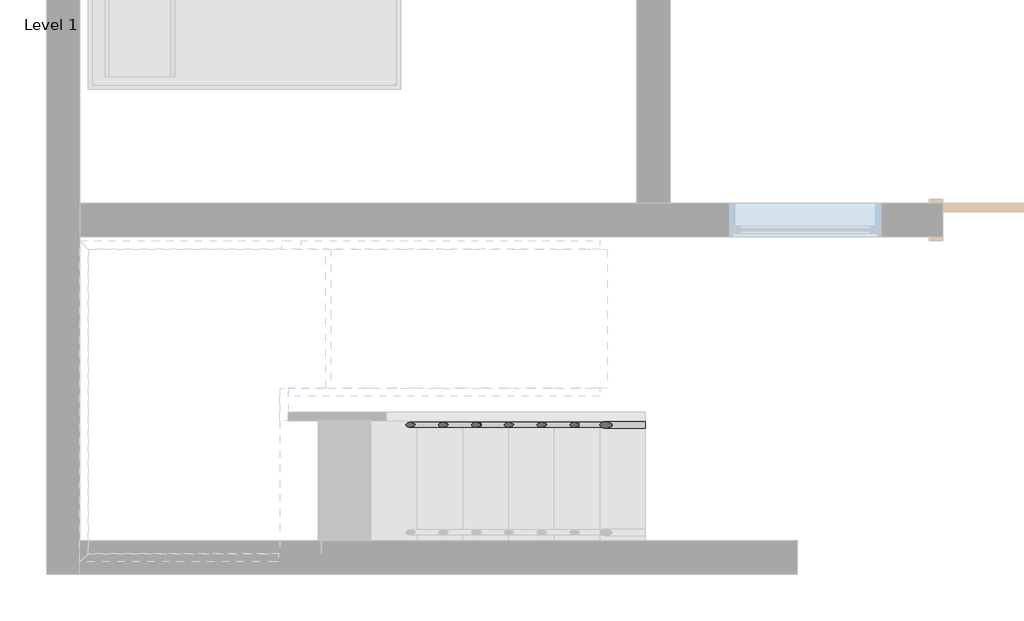
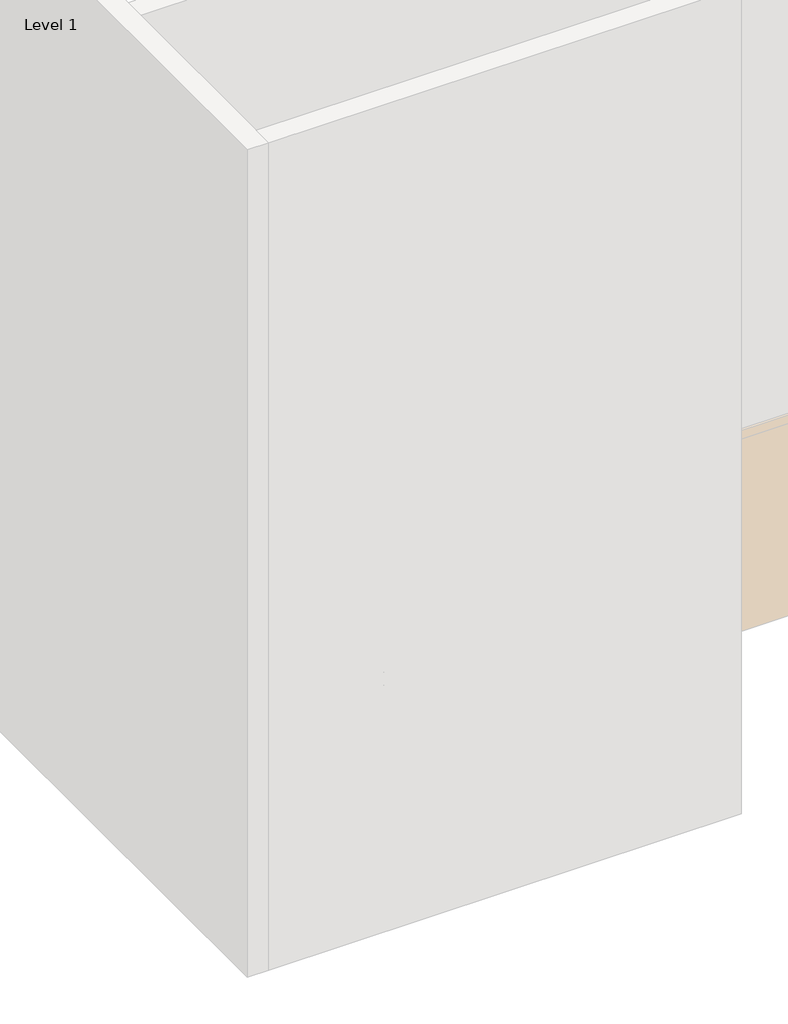
# One storey, part 2 of 4: 1 railing.
"""IFC4 building model written with IfcOpenShell, lengths in millimetres."""

from ifc_helpers import new_model, si_unit, point, frame, frame_2d, origin, place, context, project, spatial, circle_curve, ellipse_curve, trimmed, segment, composite_curve, outline, extrude, element, save
from ifc_brep_helpers import plane_surface, cylinder_surface, advanced_brep

model = new_model("IFC4")

# Units and contexts
model_context = context("Model", 3, world=origin())
ifc_project = project(units=[si_unit("LENGTHUNIT", "METRE", prefix="MILLI")], contexts=[model_context])

# Site, building, storey
site = spatial("IfcSite", under=ifc_project)
building = spatial("IfcBuilding", under=site)
storey = spatial("IfcBuildingStorey", under=building, Name="Level 1", Elevation=0.0)

# Railing
placement = place(None, origin())
element("IfcRailing", 1, ObjectType="900mm Pipe", at=placement, inside=storey, context=model_context, shape_type="SolidModel", body=[
    advanced_brep(
    [(-7153.6870075, 2206.9123547, 1050.2491997), (-7153.6870075, 2166.9123547, 1050.2491997), (-9372.8734957, 2206.9123547, 2453.687295), (-9406.680345, 2166.9123547, 2475.0671206)],
    [
        (0, 1, ellipse_curve(frame((-7153.6870075, 2186.9123547, 1050.2491997), z_axis=(1.0, 0.0, 0.0), x_axis=(0.0, 0.0, -1.0)), 23.6638438, 20.0)),
        (1, 0, ellipse_curve(frame((-7153.6870075, 2186.9123547, 1050.2491997), z_axis=(1.0, 0.0, 0.0), x_axis=(0.0, 0.0, -1.0)), 23.6638438, 20.0)),
        (2, 3, ellipse_curve(frame((-9389.7769203, 2186.9123547, 2464.3772078), z_axis=(-0.597626308985338, 0.7071067811865502, 0.3779454918484377), x_axis=(0.5976263089853449, 0.7071067811865448, -0.3779454918484371)), 28.2842712, 20.0)),
        (3, 2, ellipse_curve(frame((-9389.7769203, 2186.9123547, 2464.3772078), z_axis=(-0.597626308985338, 0.7071067811865502, 0.3779454918484377), x_axis=(0.5976263089853449, 0.7071067811865448, -0.3779454918484371)), 28.2842712, 20.0)),
        (0, 2),
        (3, 1),
    ],
    [
        plane_surface(frame((-7153.6870075, 2186.9123547, 1073.9130435), z_axis=(1.0, 0.0, 0.0), x_axis=(0.0, -1.0, 0.0))),
        plane_surface(frame((-9379.0870075, 2186.9123547, 2481.2806324), z_axis=(-0.5976263089853381, 0.7071067811865503, 0.3779454918484378), x_axis=(0.8017747781070201, 0.5270627453469418, 0.281712739610376))),
        cylinder_surface(frame((-7164.3769203, 2186.9123547, 1057.0096189), z_axis=(0.8451712313980437, 0.0, -0.5344956404098302), x_axis=(0.0, -1.0, 0.0)), 20.0),
    ],
    [
        (0, [[1, 2]]),
        (1, [[3, 4]]),
        (2, [[-1, 5, -4, 6]]),
        (2, [[-2, -6, -3, -5]]),
    ],
),
    advanced_brep(
    [(-9359.0870075, 2214.5056921, 2445.2173913), (-9399.0870075, 2180.6988429, 2445.2173913), (-9359.0870075, 2428.0117335, 2445.2173913), (-9399.0870075, 2461.8185827, 2445.2173913)],
    [
        (0, 1, ellipse_curve(frame((-9379.0870075, 2197.6022675, 2445.2173913), z_axis=(0.597626308985338, -0.7071067811865502, -0.3779454918484377), x_axis=(-0.5976263089853446, -0.7071067811865449, 0.377945491848437)), 28.2842712, 20.0)),
        (1, 0, ellipse_curve(frame((-9379.0870075, 2197.6022675, 2445.2173913), z_axis=(0.597626308985338, -0.7071067811865502, -0.3779454918484377), x_axis=(-0.5976263089853446, -0.7071067811865449, 0.377945491848437)), 28.2842712, 20.0)),
        (2, 3, ellipse_curve(frame((-9379.0870075, 2444.9151581, 2445.2173913), z_axis=(0.5976263089853451, 0.7071067811865449, 0.37794549184843684), x_axis=(0.5976263089853384, -0.70710678118655, 0.37794549184843756)), 28.2842712, 20.0)),
        (3, 2, ellipse_curve(frame((-9379.0870075, 2444.9151581, 2445.2173913), z_axis=(0.5976263089853451, 0.7071067811865449, 0.37794549184843684), x_axis=(0.5976263089853384, -0.70710678118655, 0.37794549184843756)), 28.2842712, 20.0)),
        (0, 2),
        (3, 1),
    ],
    [
        plane_surface(frame((-9379.0870075, 2186.9123547, 2465.2173913), z_axis=(0.5976263089853381, -0.7071067811865503, -0.3779454918484378), x_axis=(0.8017747781070201, 0.5270627453469418, 0.281712739610376))),
        plane_surface(frame((-9379.0870075, 2434.2252453, 2465.2173913), z_axis=(0.597626308985345, 0.7071067811865448, 0.37794549184843673), x_axis=(0.8017747781070149, -0.5270627453469473, -0.28171273961038046))),
        cylinder_surface(frame((-9379.0870075, 2186.9123547, 2445.2173913), z_axis=(0.0, -1.0, 0.0), x_axis=(-1.0, 0.0, 0.0)), 20.0),
    ],
    [
        (0, [[1, 2]]),
        (1, [[3, 4]]),
        (2, [[-1, 5, -4, 6]]),
        (2, [[-2, -6, -3, -5]]),
    ],
),
    advanced_brep(
    [(-9326.0936701, 2414.2252453, 2459.0038795), (-9359.9005194, 2454.2252453, 2437.6240539), (-7428.6870075, 2414.2252453, 3658.9448519), (-7428.6870075, 2454.2252453, 3658.9448519)],
    [
        (0, 1, ellipse_curve(frame((-9342.9970947, 2434.2252453, 2448.3139667), z_axis=(-0.5976263089853451, -0.7071067811865449, -0.37794549184843684), x_axis=(-0.5976263089853381, 0.7071067811865503, -0.3779454918484374)), 28.2842712, 20.0)),
        (1, 0, ellipse_curve(frame((-9342.9970947, 2434.2252453, 2448.3139667), z_axis=(-0.5976263089853451, -0.7071067811865449, -0.37794549184843684), x_axis=(-0.5976263089853381, 0.7071067811865503, -0.3779454918484374)), 28.2842712, 20.0)),
        (2, 3, ellipse_curve(frame((-7428.6870075, 2434.2252453, 3658.9448519), z_axis=(1.0, 0.0, 0.0), x_axis=(0.0, 0.0, -1.0)), 23.6638438, 20.0)),
        (3, 2, ellipse_curve(frame((-7428.6870075, 2434.2252453, 3658.9448519), z_axis=(1.0, 0.0, 0.0), x_axis=(0.0, 0.0, -1.0)), 23.6638438, 20.0)),
        (0, 2),
        (3, 1),
    ],
    [
        plane_surface(frame((-9353.6870075, 2434.2252453, 2465.2173913), z_axis=(-0.597626308985345, -0.7071067811865448, -0.37794549184843673), x_axis=(0.8017747781070149, -0.5270627453469473, -0.28171273961038046))),
        plane_surface(frame((-7428.6870075, 2434.2252453, 3682.6086957), z_axis=(1.0, 0.0, 0.0), x_axis=(0.0, 1.0, 0.0))),
        cylinder_surface(frame((-9342.9970947, 2434.2252453, 2448.3139667), z_axis=(-0.845171231398044, 0.0, -0.5344956404098298), x_axis=(0.0, 1.0, 0.0)), 20.0),
    ],
    [
        (0, [[1, 2]]),
        (1, [[3, 4]]),
        (2, [[-1, 5, -4, 6]]),
        (2, [[-2, -6, -3, -5]]),
    ],
),
    advanced_brep(
    [(-7153.6870075, 2171.9123547, 931.1651606), (-7153.6870075, 2201.9123547, 931.1651606), (-9358.0320973, 2171.9123547, 2325.2173913), (-9358.0320973, 2201.9123547, 2325.2173913), (-9394.0870075, 2171.9123547, 2325.2173913), (-9364.0870075, 2201.9123547, 2325.2173913), (-9394.0870075, 2449.2252453, 2325.2173913), (-9364.0870075, 2419.2252453, 2325.2173913), (-9349.3419178, 2449.2252453, 2325.2173913), (-9349.3419178, 2419.2252453, 2325.2173913), (-7428.6870075, 2449.2252453, 3539.8608128), (-7428.6870075, 2419.2252453, 3539.8608128)],
    [
        (0, 1, ellipse_curve(frame((-7153.6870075, 2186.9123547, 931.1651606), z_axis=(1.0, 0.0, 0.0), x_axis=(0.0, 0.0, -1.0)), 17.7478828, 15.0)),
        (1, 0, ellipse_curve(frame((-7153.6870075, 2186.9123547, 931.1651606), z_axis=(1.0, 0.0, 0.0), x_axis=(0.0, 0.0, -1.0)), 17.7478828, 15.0)),
        (0, 2),
        (2, 3, ellipse_curve(frame((-9358.0320973, 2186.9123547, 2325.2173913), z_axis=(0.9605132043335073, 0.0, -0.2782344053149754), x_axis=(-0.27823440531497523, 0.0, -0.9605132043335072)), 15.6166515, 15.0)),
        (3, 1),
        (3, 2, ellipse_curve(frame((-9358.0320973, 2186.9123547, 2325.2173913), z_axis=(0.9605132043335073, 0.0, -0.2782344053149754), x_axis=(-0.27823440531497523, 0.0, -0.9605132043335072)), 15.6166515, 15.0)),
        (2, 4),
        (4, 5, ellipse_curve(frame((-9379.0870075, 2186.9123547, 2325.2173913), z_axis=(0.7071067811865445, -0.7071067811865507, 0.0), x_axis=(0.7071067811865506, 0.7071067811865445, 0.0)), 21.2132034, 15.0)),
        (5, 3),
        (5, 4, ellipse_curve(frame((-9379.0870075, 2186.9123547, 2325.2173913), z_axis=(0.7071067811865445, -0.7071067811865507, 0.0), x_axis=(0.7071067811865506, 0.7071067811865445, 0.0)), 21.2132034, 15.0)),
        (4, 6),
        (6, 7, ellipse_curve(frame((-9379.0870075, 2434.2252453, 2325.2173913), z_axis=(-0.7071067811865506, -0.7071067811865442, 0.0), x_axis=(0.7071067811865441, -0.707106781186551, 0.0)), 21.2132034, 15.0)),
        (7, 5),
        (7, 6, ellipse_curve(frame((-9379.0870075, 2434.2252453, 2325.2173913), z_axis=(-0.7071067811865506, -0.7071067811865442, 0.0), x_axis=(0.7071067811865441, -0.707106781186551, 0.0)), 21.2132034, 15.0)),
        (6, 8),
        (8, 9, ellipse_curve(frame((-9349.3419178, 2434.2252453, 2325.2173913), z_axis=(-0.9605132043335073, 0.0, -0.2782344053149753), x_axis=(-0.2782344053149759, 0.0, 0.9605132043335072)), 15.6166515, 15.0)),
        (9, 7),
        (9, 8, ellipse_curve(frame((-9349.3419178, 2434.2252453, 2325.2173913), z_axis=(-0.9605132043335073, 0.0, -0.2782344053149753), x_axis=(-0.2782344053149759, 0.0, 0.9605132043335072)), 15.6166515, 15.0)),
        (10, 11, ellipse_curve(frame((-7428.6870075, 2434.2252453, 3539.8608128), z_axis=(1.0, 0.0, 0.0), x_axis=(0.0, 0.0, -1.0)), 17.7478828, 15.0)),
        (11, 10, ellipse_curve(frame((-7428.6870075, 2434.2252453, 3539.8608128), z_axis=(1.0, 0.0, 0.0), x_axis=(0.0, 0.0, -1.0)), 17.7478828, 15.0)),
        (8, 10),
        (11, 9),
    ],
    [
        plane_surface(frame((-7153.6870075, 2186.9123547, 948.9130435), z_axis=(1.0, 0.0, 0.0), x_axis=(0.0, -1.0, 0.0))),
        cylinder_surface(frame((-7161.7044421, 2186.9123547, 936.235475), z_axis=(0.8451712313980438, 0.0, -0.5344956404098299), x_axis=(0.0, 1.0, 0.0)), 15.0),
        cylinder_surface(frame((-9353.6870075, 2186.9123547, 2325.2173913), z_axis=(1.0, 0.0, 0.0), x_axis=(0.0, 1.0, 0.0)), 15.0),
        cylinder_surface(frame((-9379.0870075, 2186.9123547, 2325.2173913), z_axis=(0.0, -1.0, 0.0), x_axis=(1.0, 0.0, 0.0)), 15.0),
        cylinder_surface(frame((-9379.0870075, 2434.2252453, 2325.2173913), z_axis=(-1.0, 0.0, 0.0), x_axis=(0.0, -1.0, 0.0)), 15.0),
        plane_surface(frame((-7428.6870075, 2434.2252453, 3557.6086957), z_axis=(1.0, 0.0, 0.0), x_axis=(0.0, 1.0, 0.0))),
        cylinder_surface(frame((-9345.6695729, 2434.2252453, 2327.5398228), z_axis=(-0.845171231398044, 0.0, -0.5344956404098297), x_axis=(0.0, -1.0, 0.0)), 15.0),
    ],
    [
        (0, [[1, 2]]),
        (1, [[-1, 3, 4, 5]]),
        (1, [[-2, -5, 6, -3]]),
        (2, [[-4, 7, 8, 9]]),
        (2, [[-6, -9, 10, -7]]),
        (3, [[-8, 11, 12, 13]]),
        (3, [[-10, -13, 14, -11]]),
        (4, [[-12, 15, 16, 17]]),
        (4, [[-14, -17, 18, -15]]),
        (5, [[19, 20]]),
        (6, [[-16, 21, -20, 22]]),
        (6, [[-18, -22, -19, -21]]),
    ],
),
    advanced_brep(
    [(-7153.6870075, 2171.9123547, 806.1651606), (-7153.6870075, 2201.9123547, 806.1651606), (-9358.0320973, 2171.9123547, 2200.2173913), (-9358.0320973, 2201.9123547, 2200.2173913), (-9394.0870075, 2171.9123547, 2200.2173913), (-9364.0870075, 2201.9123547, 2200.2173913), (-9394.0870075, 2449.2252453, 2200.2173913), (-9364.0870075, 2419.2252453, 2200.2173913), (-9349.3419178, 2449.2252453, 2200.2173913), (-9349.3419178, 2419.2252453, 2200.2173913), (-7428.6870075, 2449.2252453, 3414.8608128), (-7428.6870075, 2419.2252453, 3414.8608128)],
    [
        (0, 1, ellipse_curve(frame((-7153.6870075, 2186.9123547, 806.1651606), z_axis=(1.0, 0.0, 0.0), x_axis=(0.0, 0.0, -1.0)), 17.7478828, 15.0)),
        (1, 0, ellipse_curve(frame((-7153.6870075, 2186.9123547, 806.1651606), z_axis=(1.0, 0.0, 0.0), x_axis=(0.0, 0.0, -1.0)), 17.7478828, 15.0)),
        (0, 2),
        (2, 3, ellipse_curve(frame((-9358.0320973, 2186.9123547, 2200.2173913), z_axis=(0.9605132043335073, 0.0, -0.2782344053149754), x_axis=(-0.27823440531497523, 0.0, -0.9605132043335072)), 15.6166515, 15.0)),
        (3, 1),
        (3, 2, ellipse_curve(frame((-9358.0320973, 2186.9123547, 2200.2173913), z_axis=(0.9605132043335073, 0.0, -0.2782344053149754), x_axis=(-0.27823440531497523, 0.0, -0.9605132043335072)), 15.6166515, 15.0)),
        (2, 4),
        (4, 5, ellipse_curve(frame((-9379.0870075, 2186.9123547, 2200.2173913), z_axis=(0.7071067811865445, -0.7071067811865507, 0.0), x_axis=(0.7071067811865506, 0.7071067811865445, 0.0)), 21.2132034, 15.0)),
        (5, 3),
        (5, 4, ellipse_curve(frame((-9379.0870075, 2186.9123547, 2200.2173913), z_axis=(0.7071067811865445, -0.7071067811865507, 0.0), x_axis=(0.7071067811865506, 0.7071067811865445, 0.0)), 21.2132034, 15.0)),
        (4, 6),
        (6, 7, ellipse_curve(frame((-9379.0870075, 2434.2252453, 2200.2173913), z_axis=(-0.7071067811865506, -0.7071067811865442, 0.0), x_axis=(0.7071067811865441, -0.707106781186551, 0.0)), 21.2132034, 15.0)),
        (7, 5),
        (7, 6, ellipse_curve(frame((-9379.0870075, 2434.2252453, 2200.2173913), z_axis=(-0.7071067811865506, -0.7071067811865442, 0.0), x_axis=(0.7071067811865441, -0.707106781186551, 0.0)), 21.2132034, 15.0)),
        (6, 8),
        (8, 9, ellipse_curve(frame((-9349.3419178, 2434.2252453, 2200.2173913), z_axis=(-0.9605132043335073, 0.0, -0.2782344053149754), x_axis=(-0.2782344053149758, 0.0, 0.9605132043335072)), 15.6166515, 15.0)),
        (9, 7),
        (9, 8, ellipse_curve(frame((-9349.3419178, 2434.2252453, 2200.2173913), z_axis=(-0.9605132043335073, 0.0, -0.2782344053149754), x_axis=(-0.2782344053149758, 0.0, 0.9605132043335072)), 15.6166515, 15.0)),
        (10, 11, ellipse_curve(frame((-7428.6870075, 2434.2252453, 3414.8608128), z_axis=(1.0, 0.0, 0.0), x_axis=(0.0, 0.0, -1.0)), 17.7478828, 15.0)),
        (11, 10, ellipse_curve(frame((-7428.6870075, 2434.2252453, 3414.8608128), z_axis=(1.0, 0.0, 0.0), x_axis=(0.0, 0.0, -1.0)), 17.7478828, 15.0)),
        (8, 10),
        (11, 9),
    ],
    [
        plane_surface(frame((-7153.6870075, 2186.9123547, 823.9130435), z_axis=(1.0, 0.0, 0.0), x_axis=(0.0, -1.0, 0.0))),
        cylinder_surface(frame((-7161.7044421, 2186.9123547, 811.235475), z_axis=(0.8451712313980438, 0.0, -0.5344956404098299), x_axis=(0.0, 1.0, 0.0)), 15.0),
        cylinder_surface(frame((-9353.6870075, 2186.9123547, 2200.2173913), z_axis=(1.0, 0.0, 0.0), x_axis=(0.0, 1.0, 0.0)), 15.0),
        cylinder_surface(frame((-9379.0870075, 2186.9123547, 2200.2173913), z_axis=(0.0, -1.0, 0.0), x_axis=(1.0, 0.0, 0.0)), 15.0),
        cylinder_surface(frame((-9379.0870075, 2434.2252453, 2200.2173913), z_axis=(-1.0, 0.0, 0.0), x_axis=(0.0, -1.0, 0.0)), 15.0),
        plane_surface(frame((-7428.6870075, 2434.2252453, 3432.6086957), z_axis=(1.0, 0.0, 0.0), x_axis=(0.0, 1.0, 0.0))),
        cylinder_surface(frame((-9345.6695729, 2434.2252453, 2202.5398228), z_axis=(-0.845171231398044, 0.0, -0.5344956404098298), x_axis=(0.0, -1.0, 0.0)), 15.0),
    ],
    [
        (0, [[1, 2]]),
        (1, [[-1, 3, 4, 5]]),
        (1, [[-2, -5, 6, -3]]),
        (2, [[-4, 7, 8, 9]]),
        (2, [[-6, -9, 10, -7]]),
        (3, [[-8, 11, 12, 13]]),
        (3, [[-10, -13, 14, -11]]),
        (4, [[-12, 15, 16, 17]]),
        (4, [[-14, -17, 18, -15]]),
        (5, [[19, 20]]),
        (6, [[-16, 21, -20, 22]]),
        (6, [[-18, -22, -19, -21]]),
    ],
),
    advanced_brep(
    [(-7153.6870075, 2171.9123547, 681.1651606), (-7153.6870075, 2201.9123547, 681.1651606), (-9358.0320973, 2171.9123547, 2075.2173913), (-9358.0320973, 2201.9123547, 2075.2173913), (-9394.0870075, 2171.9123547, 2075.2173913), (-9364.0870075, 2201.9123547, 2075.2173913), (-9394.0870075, 2449.2252453, 2075.2173913), (-9364.0870075, 2419.2252453, 2075.2173913), (-9349.3419178, 2449.2252453, 2075.2173913), (-9349.3419178, 2419.2252453, 2075.2173913), (-7428.6870075, 2449.2252453, 3289.8608128), (-7428.6870075, 2419.2252453, 3289.8608128)],
    [
        (0, 1, ellipse_curve(frame((-7153.6870075, 2186.9123547, 681.1651606), z_axis=(1.0, 0.0, 0.0), x_axis=(0.0, 0.0, -1.0)), 17.7478828, 15.0)),
        (1, 0, ellipse_curve(frame((-7153.6870075, 2186.9123547, 681.1651606), z_axis=(1.0, 0.0, 0.0), x_axis=(0.0, 0.0, -1.0)), 17.7478828, 15.0)),
        (0, 2),
        (2, 3, ellipse_curve(frame((-9358.0320973, 2186.9123547, 2075.2173913), z_axis=(0.9605132043335073, 0.0, -0.2782344053149754), x_axis=(-0.27823440531497523, 0.0, -0.9605132043335072)), 15.6166515, 15.0)),
        (3, 1),
        (3, 2, ellipse_curve(frame((-9358.0320973, 2186.9123547, 2075.2173913), z_axis=(0.9605132043335073, 0.0, -0.2782344053149754), x_axis=(-0.27823440531497523, 0.0, -0.9605132043335072)), 15.6166515, 15.0)),
        (2, 4),
        (4, 5, ellipse_curve(frame((-9379.0870075, 2186.9123547, 2075.2173913), z_axis=(0.7071067811865445, -0.7071067811865507, 0.0), x_axis=(0.7071067811865506, 0.7071067811865445, 0.0)), 21.2132034, 15.0)),
        (5, 3),
        (5, 4, ellipse_curve(frame((-9379.0870075, 2186.9123547, 2075.2173913), z_axis=(0.7071067811865445, -0.7071067811865507, 0.0), x_axis=(0.7071067811865506, 0.7071067811865445, 0.0)), 21.2132034, 15.0)),
        (4, 6),
        (6, 7, ellipse_curve(frame((-9379.0870075, 2434.2252453, 2075.2173913), z_axis=(-0.7071067811865506, -0.7071067811865442, 0.0), x_axis=(0.7071067811865441, -0.707106781186551, 0.0)), 21.2132034, 15.0)),
        (7, 5),
        (7, 6, ellipse_curve(frame((-9379.0870075, 2434.2252453, 2075.2173913), z_axis=(-0.7071067811865506, -0.7071067811865442, 0.0), x_axis=(0.7071067811865441, -0.707106781186551, 0.0)), 21.2132034, 15.0)),
        (6, 8),
        (8, 9, ellipse_curve(frame((-9349.3419178, 2434.2252453, 2075.2173913), z_axis=(-0.9605132043335073, 0.0, -0.2782344053149754), x_axis=(-0.2782344053149758, 0.0, 0.9605132043335072)), 15.6166515, 15.0)),
        (9, 7),
        (9, 8, ellipse_curve(frame((-9349.3419178, 2434.2252453, 2075.2173913), z_axis=(-0.9605132043335073, 0.0, -0.2782344053149754), x_axis=(-0.2782344053149758, 0.0, 0.9605132043335072)), 15.6166515, 15.0)),
        (10, 11, ellipse_curve(frame((-7428.6870075, 2434.2252453, 3289.8608128), z_axis=(1.0, 0.0, 0.0), x_axis=(0.0, 0.0, -1.0)), 17.7478828, 15.0)),
        (11, 10, ellipse_curve(frame((-7428.6870075, 2434.2252453, 3289.8608128), z_axis=(1.0, 0.0, 0.0), x_axis=(0.0, 0.0, -1.0)), 17.7478828, 15.0)),
        (8, 10),
        (11, 9),
    ],
    [
        plane_surface(frame((-7153.6870075, 2186.9123547, 698.9130435), z_axis=(1.0, 0.0, 0.0), x_axis=(0.0, -1.0, 0.0))),
        cylinder_surface(frame((-7161.7044421, 2186.9123547, 686.235475), z_axis=(0.8451712313980438, 0.0, -0.5344956404098299), x_axis=(0.0, 1.0, 0.0)), 15.0),
        cylinder_surface(frame((-9353.6870075, 2186.9123547, 2075.2173913), z_axis=(1.0, 0.0, 0.0), x_axis=(0.0, 1.0, 0.0)), 15.0),
        cylinder_surface(frame((-9379.0870075, 2186.9123547, 2075.2173913), z_axis=(0.0, -1.0, 0.0), x_axis=(1.0, 0.0, 0.0)), 15.0),
        cylinder_surface(frame((-9379.0870075, 2434.2252453, 2075.2173913), z_axis=(-1.0, 0.0, 0.0), x_axis=(0.0, -1.0, 0.0)), 15.0),
        plane_surface(frame((-7428.6870075, 2434.2252453, 3307.6086957), z_axis=(1.0, 0.0, 0.0), x_axis=(0.0, 1.0, 0.0))),
        cylinder_surface(frame((-9345.6695729, 2434.2252453, 2077.5398228), z_axis=(-0.845171231398044, 0.0, -0.5344956404098299), x_axis=(0.0, -1.0, 0.0)), 15.0),
    ],
    [
        (0, [[1, 2]]),
        (1, [[-1, 3, 4, 5]]),
        (1, [[-2, -5, 6, -3]]),
        (2, [[-4, 7, 8, 9]]),
        (2, [[-6, -9, 10, -7]]),
        (3, [[-8, 11, 12, 13]]),
        (3, [[-10, -13, 14, -11]]),
        (4, [[-12, 15, 16, 17]]),
        (4, [[-14, -17, 18, -15]]),
        (5, [[19, 20]]),
        (6, [[-16, 21, -20, 22]]),
        (6, [[-18, -22, -19, -21]]),
    ],
),
    advanced_brep(
    [(-7153.6870075, 2171.9123547, 556.1651606), (-7153.6870075, 2201.9123547, 556.1651606), (-9358.0320973, 2171.9123547, 1950.2173913), (-9358.0320973, 2201.9123547, 1950.2173913), (-9394.0870075, 2171.9123547, 1950.2173913), (-9364.0870075, 2201.9123547, 1950.2173913), (-9394.0870075, 2449.2252453, 1950.2173913), (-9364.0870075, 2419.2252453, 1950.2173913), (-9349.3419178, 2449.2252453, 1950.2173913), (-9349.3419178, 2419.2252453, 1950.2173913), (-7428.6870075, 2449.2252453, 3164.8608128), (-7428.6870075, 2419.2252453, 3164.8608128)],
    [
        (0, 1, ellipse_curve(frame((-7153.6870075, 2186.9123547, 556.1651606), z_axis=(1.0, 0.0, 0.0), x_axis=(0.0, 0.0, -1.0)), 17.7478828, 15.0)),
        (1, 0, ellipse_curve(frame((-7153.6870075, 2186.9123547, 556.1651606), z_axis=(1.0, 0.0, 0.0), x_axis=(0.0, 0.0, -1.0)), 17.7478828, 15.0)),
        (0, 2),
        (2, 3, ellipse_curve(frame((-9358.0320973, 2186.9123547, 1950.2173913), z_axis=(0.9605132043335073, 0.0, -0.2782344053149754), x_axis=(-0.27823440531497523, 0.0, -0.9605132043335072)), 15.6166515, 15.0)),
        (3, 1),
        (3, 2, ellipse_curve(frame((-9358.0320973, 2186.9123547, 1950.2173913), z_axis=(0.9605132043335073, 0.0, -0.2782344053149754), x_axis=(-0.27823440531497523, 0.0, -0.9605132043335072)), 15.6166515, 15.0)),
        (2, 4),
        (4, 5, ellipse_curve(frame((-9379.0870075, 2186.9123547, 1950.2173913), z_axis=(0.7071067811865445, -0.7071067811865507, 0.0), x_axis=(0.7071067811865506, 0.7071067811865445, 0.0)), 21.2132034, 15.0)),
        (5, 3),
        (5, 4, ellipse_curve(frame((-9379.0870075, 2186.9123547, 1950.2173913), z_axis=(0.7071067811865445, -0.7071067811865507, 0.0), x_axis=(0.7071067811865506, 0.7071067811865445, 0.0)), 21.2132034, 15.0)),
        (4, 6),
        (6, 7, ellipse_curve(frame((-9379.0870075, 2434.2252453, 1950.2173913), z_axis=(-0.7071067811865506, -0.7071067811865442, 0.0), x_axis=(0.7071067811865441, -0.707106781186551, 0.0)), 21.2132034, 15.0)),
        (7, 5),
        (7, 6, ellipse_curve(frame((-9379.0870075, 2434.2252453, 1950.2173913), z_axis=(-0.7071067811865506, -0.7071067811865442, 0.0), x_axis=(0.7071067811865441, -0.707106781186551, 0.0)), 21.2132034, 15.0)),
        (6, 8),
        (8, 9, ellipse_curve(frame((-9349.3419178, 2434.2252453, 1950.2173913), z_axis=(-0.9605132043335073, 0.0, -0.2782344053149754), x_axis=(-0.2782344053149758, 0.0, 0.9605132043335072)), 15.6166515, 15.0)),
        (9, 7),
        (9, 8, ellipse_curve(frame((-9349.3419178, 2434.2252453, 1950.2173913), z_axis=(-0.9605132043335073, 0.0, -0.2782344053149754), x_axis=(-0.2782344053149758, 0.0, 0.9605132043335072)), 15.6166515, 15.0)),
        (10, 11, ellipse_curve(frame((-7428.6870075, 2434.2252453, 3164.8608128), z_axis=(1.0, 0.0, 0.0), x_axis=(0.0, 0.0, -1.0)), 17.7478828, 15.0)),
        (11, 10, ellipse_curve(frame((-7428.6870075, 2434.2252453, 3164.8608128), z_axis=(1.0, 0.0, 0.0), x_axis=(0.0, 0.0, -1.0)), 17.7478828, 15.0)),
        (8, 10),
        (11, 9),
    ],
    [
        plane_surface(frame((-7153.6870075, 2186.9123547, 573.9130435), z_axis=(1.0, 0.0, 0.0), x_axis=(0.0, -1.0, 0.0))),
        cylinder_surface(frame((-7161.7044421, 2186.9123547, 561.235475), z_axis=(0.8451712313980438, 0.0, -0.5344956404098299), x_axis=(0.0, 1.0, 0.0)), 15.0),
        cylinder_surface(frame((-9353.6870075, 2186.9123547, 1950.2173913), z_axis=(1.0, 0.0, 0.0), x_axis=(0.0, 1.0, 0.0)), 15.0),
        cylinder_surface(frame((-9379.0870075, 2186.9123547, 1950.2173913), z_axis=(0.0, -1.0, 0.0), x_axis=(1.0, 0.0, 0.0)), 15.0),
        cylinder_surface(frame((-9379.0870075, 2434.2252453, 1950.2173913), z_axis=(-1.0, 0.0, 0.0), x_axis=(0.0, -1.0, 0.0)), 15.0),
        plane_surface(frame((-7428.6870075, 2434.2252453, 3182.6086957), z_axis=(1.0, 0.0, 0.0), x_axis=(0.0, 1.0, 0.0))),
        cylinder_surface(frame((-9345.6695729, 2434.2252453, 1952.5398228), z_axis=(-0.845171231398044, 0.0, -0.5344956404098298), x_axis=(0.0, -1.0, 0.0)), 15.0),
    ],
    [
        (0, [[1, 2]]),
        (1, [[-1, 3, 4, 5]]),
        (1, [[-2, -5, 6, -3]]),
        (2, [[-4, 7, 8, 9]]),
        (2, [[-6, -9, 10, -7]]),
        (3, [[-8, 11, 12, 13]]),
        (3, [[-10, -13, 14, -11]]),
        (4, [[-12, 15, 16, 17]]),
        (4, [[-14, -17, 18, -15]]),
        (5, [[19, 20]]),
        (6, [[-16, 21, -20, 22]]),
        (6, [[-18, -22, -19, -21]]),
    ],
),
    advanced_brep(
    [(-7153.6870075, 2171.9123547, 431.1651606), (-7153.6870075, 2201.9123547, 431.1651606), (-9358.0320973, 2171.9123547, 1825.2173913), (-9358.0320973, 2201.9123547, 1825.2173913), (-9394.0870075, 2171.9123547, 1825.2173913), (-9364.0870075, 2201.9123547, 1825.2173913), (-9394.0870075, 2449.2252453, 1825.2173913), (-9364.0870075, 2419.2252453, 1825.2173913), (-9349.3419178, 2449.2252453, 1825.2173913), (-9349.3419178, 2419.2252453, 1825.2173913), (-7428.6870075, 2449.2252453, 3039.8608128), (-7428.6870075, 2419.2252453, 3039.8608128)],
    [
        (0, 1, ellipse_curve(frame((-7153.6870075, 2186.9123547, 431.1651606), z_axis=(1.0, 0.0, 0.0), x_axis=(0.0, 0.0, -1.0)), 17.7478828, 15.0)),
        (1, 0, ellipse_curve(frame((-7153.6870075, 2186.9123547, 431.1651606), z_axis=(1.0, 0.0, 0.0), x_axis=(0.0, 0.0, -1.0)), 17.7478828, 15.0)),
        (0, 2),
        (2, 3, ellipse_curve(frame((-9358.0320973, 2186.9123547, 1825.2173913), z_axis=(0.9605132043335073, 0.0, -0.2782344053149754), x_axis=(-0.27823440531497523, 0.0, -0.9605132043335072)), 15.6166515, 15.0)),
        (3, 1),
        (3, 2, ellipse_curve(frame((-9358.0320973, 2186.9123547, 1825.2173913), z_axis=(0.9605132043335073, 0.0, -0.2782344053149754), x_axis=(-0.27823440531497523, 0.0, -0.9605132043335072)), 15.6166515, 15.0)),
        (2, 4),
        (4, 5, ellipse_curve(frame((-9379.0870075, 2186.9123547, 1825.2173913), z_axis=(0.7071067811865445, -0.7071067811865507, 0.0), x_axis=(0.7071067811865506, 0.7071067811865445, 0.0)), 21.2132034, 15.0)),
        (5, 3),
        (5, 4, ellipse_curve(frame((-9379.0870075, 2186.9123547, 1825.2173913), z_axis=(0.7071067811865445, -0.7071067811865507, 0.0), x_axis=(0.7071067811865506, 0.7071067811865445, 0.0)), 21.2132034, 15.0)),
        (4, 6),
        (6, 7, ellipse_curve(frame((-9379.0870075, 2434.2252453, 1825.2173913), z_axis=(-0.7071067811865506, -0.7071067811865442, 0.0), x_axis=(0.7071067811865441, -0.707106781186551, 0.0)), 21.2132034, 15.0)),
        (7, 5),
        (7, 6, ellipse_curve(frame((-9379.0870075, 2434.2252453, 1825.2173913), z_axis=(-0.7071067811865506, -0.7071067811865442, 0.0), x_axis=(0.7071067811865441, -0.707106781186551, 0.0)), 21.2132034, 15.0)),
        (6, 8),
        (8, 9, ellipse_curve(frame((-9349.3419178, 2434.2252453, 1825.2173913), z_axis=(-0.9605132043335073, 0.0, -0.2782344053149753), x_axis=(-0.2782344053149759, 0.0, 0.9605132043335072)), 15.6166515, 15.0)),
        (9, 7),
        (9, 8, ellipse_curve(frame((-9349.3419178, 2434.2252453, 1825.2173913), z_axis=(-0.9605132043335073, 0.0, -0.2782344053149753), x_axis=(-0.2782344053149759, 0.0, 0.9605132043335072)), 15.6166515, 15.0)),
        (10, 11, ellipse_curve(frame((-7428.6870075, 2434.2252453, 3039.8608128), z_axis=(1.0, 0.0, 0.0), x_axis=(0.0, 0.0, -1.0)), 17.7478828, 15.0)),
        (11, 10, ellipse_curve(frame((-7428.6870075, 2434.2252453, 3039.8608128), z_axis=(1.0, 0.0, 0.0), x_axis=(0.0, 0.0, -1.0)), 17.7478828, 15.0)),
        (8, 10),
        (11, 9),
    ],
    [
        plane_surface(frame((-7153.6870075, 2186.9123547, 448.9130435), z_axis=(1.0, 0.0, 0.0), x_axis=(0.0, -1.0, 0.0))),
        cylinder_surface(frame((-7161.7044421, 2186.9123547, 436.235475), z_axis=(0.8451712313980438, 0.0, -0.5344956404098299), x_axis=(0.0, 1.0, 0.0)), 15.0),
        cylinder_surface(frame((-9353.6870075, 2186.9123547, 1825.2173913), z_axis=(1.0, 0.0, 0.0), x_axis=(0.0, 1.0, 0.0)), 15.0),
        cylinder_surface(frame((-9379.0870075, 2186.9123547, 1825.2173913), z_axis=(0.0, -1.0, 0.0), x_axis=(1.0, 0.0, 0.0)), 15.0),
        cylinder_surface(frame((-9379.0870075, 2434.2252453, 1825.2173913), z_axis=(-1.0, 0.0, 0.0), x_axis=(0.0, -1.0, 0.0)), 15.0),
        plane_surface(frame((-7428.6870075, 2434.2252453, 3057.6086957), z_axis=(1.0, 0.0, 0.0), x_axis=(0.0, 1.0, 0.0))),
        cylinder_surface(frame((-9345.6695729, 2434.2252453, 1827.5398228), z_axis=(-0.845171231398044, 0.0, -0.5344956404098297), x_axis=(0.0, -1.0, 0.0)), 15.0),
    ],
    [
        (0, [[1, 2]]),
        (1, [[-1, 3, 4, 5]]),
        (1, [[-2, -5, 6, -3]]),
        (2, [[-4, 7, 8, 9]]),
        (2, [[-6, -9, 10, -7]]),
        (3, [[-8, 11, 12, 13]]),
        (3, [[-10, -13, 14, -11]]),
        (4, [[-12, 15, 16, 17]]),
        (4, [[-14, -17, 18, -15]]),
        (5, [[19, 20]]),
        (6, [[-16, 21, -20, 22]]),
        (6, [[-18, -22, -19, -21]]),
    ],
),
    advanced_brep(
    [(-7153.6870075, 2171.9123547, 306.1651606), (-7153.6870075, 2201.9123547, 306.1651606), (-9358.0320973, 2171.9123547, 1700.2173913), (-9358.0320973, 2201.9123547, 1700.2173913), (-9394.0870075, 2171.9123547, 1700.2173913), (-9364.0870075, 2201.9123547, 1700.2173913), (-9394.0870075, 2449.2252453, 1700.2173913), (-9364.0870075, 2419.2252453, 1700.2173913), (-9349.3419178, 2449.2252453, 1700.2173913), (-9349.3419178, 2419.2252453, 1700.2173913), (-7428.6870075, 2449.2252453, 2914.8608128), (-7428.6870075, 2419.2252453, 2914.8608128)],
    [
        (0, 1, ellipse_curve(frame((-7153.6870075, 2186.9123547, 306.1651606), z_axis=(1.0, 0.0, 0.0), x_axis=(0.0, 0.0, -1.0)), 17.7478828, 15.0)),
        (1, 0, ellipse_curve(frame((-7153.6870075, 2186.9123547, 306.1651606), z_axis=(1.0, 0.0, 0.0), x_axis=(0.0, 0.0, -1.0)), 17.7478828, 15.0)),
        (0, 2),
        (2, 3, ellipse_curve(frame((-9358.0320973, 2186.9123547, 1700.2173913), z_axis=(0.9605132043335073, 0.0, -0.2782344053149754), x_axis=(-0.27823440531497523, 0.0, -0.9605132043335072)), 15.6166515, 15.0)),
        (3, 1),
        (3, 2, ellipse_curve(frame((-9358.0320973, 2186.9123547, 1700.2173913), z_axis=(0.9605132043335073, 0.0, -0.2782344053149754), x_axis=(-0.27823440531497523, 0.0, -0.9605132043335072)), 15.6166515, 15.0)),
        (2, 4),
        (4, 5, ellipse_curve(frame((-9379.0870075, 2186.9123547, 1700.2173913), z_axis=(0.7071067811865445, -0.7071067811865507, 0.0), x_axis=(0.7071067811865506, 0.7071067811865445, 0.0)), 21.2132034, 15.0)),
        (5, 3),
        (5, 4, ellipse_curve(frame((-9379.0870075, 2186.9123547, 1700.2173913), z_axis=(0.7071067811865445, -0.7071067811865507, 0.0), x_axis=(0.7071067811865506, 0.7071067811865445, 0.0)), 21.2132034, 15.0)),
        (4, 6),
        (6, 7, ellipse_curve(frame((-9379.0870075, 2434.2252453, 1700.2173913), z_axis=(-0.7071067811865506, -0.7071067811865442, 0.0), x_axis=(0.7071067811865441, -0.707106781186551, 0.0)), 21.2132034, 15.0)),
        (7, 5),
        (7, 6, ellipse_curve(frame((-9379.0870075, 2434.2252453, 1700.2173913), z_axis=(-0.7071067811865506, -0.7071067811865442, 0.0), x_axis=(0.7071067811865441, -0.707106781186551, 0.0)), 21.2132034, 15.0)),
        (6, 8),
        (8, 9, ellipse_curve(frame((-9349.3419178, 2434.2252453, 1700.2173913), z_axis=(-0.9605132043335073, 0.0, -0.2782344053149754), x_axis=(-0.2782344053149758, 0.0, 0.9605132043335072)), 15.6166515, 15.0)),
        (9, 7),
        (9, 8, ellipse_curve(frame((-9349.3419178, 2434.2252453, 1700.2173913), z_axis=(-0.9605132043335073, 0.0, -0.2782344053149754), x_axis=(-0.2782344053149758, 0.0, 0.9605132043335072)), 15.6166515, 15.0)),
        (10, 11, ellipse_curve(frame((-7428.6870075, 2434.2252453, 2914.8608128), z_axis=(1.0, 0.0, 0.0), x_axis=(0.0, 0.0, -1.0)), 17.7478828, 15.0)),
        (11, 10, ellipse_curve(frame((-7428.6870075, 2434.2252453, 2914.8608128), z_axis=(1.0, 0.0, 0.0), x_axis=(0.0, 0.0, -1.0)), 17.7478828, 15.0)),
        (8, 10),
        (11, 9),
    ],
    [
        plane_surface(frame((-7153.6870075, 2186.9123547, 323.9130435), z_axis=(1.0, 0.0, 0.0), x_axis=(0.0, -1.0, 0.0))),
        cylinder_surface(frame((-7161.7044421, 2186.9123547, 311.235475), z_axis=(0.8451712313980438, 0.0, -0.5344956404098299), x_axis=(0.0, 1.0, 0.0)), 15.0),
        cylinder_surface(frame((-9353.6870075, 2186.9123547, 1700.2173913), z_axis=(1.0, 0.0, 0.0), x_axis=(0.0, 1.0, 0.0)), 15.0),
        cylinder_surface(frame((-9379.0870075, 2186.9123547, 1700.2173913), z_axis=(0.0, -1.0, 0.0), x_axis=(1.0, 0.0, 0.0)), 15.0),
        cylinder_surface(frame((-9379.0870075, 2434.2252453, 1700.2173913), z_axis=(-1.0, 0.0, 0.0), x_axis=(0.0, -1.0, 0.0)), 15.0),
        plane_surface(frame((-7428.6870075, 2434.2252453, 2932.6086957), z_axis=(1.0, 0.0, 0.0), x_axis=(0.0, 1.0, 0.0))),
        cylinder_surface(frame((-9345.6695729, 2434.2252453, 1702.5398228), z_axis=(-0.845171231398044, 0.0, -0.5344956404098298), x_axis=(0.0, -1.0, 0.0)), 15.0),
    ],
    [
        (0, [[1, 2]]),
        (1, [[-1, 3, 4, 5]]),
        (1, [[-2, -5, 6, -3]]),
        (2, [[-4, 7, 8, 9]]),
        (2, [[-6, -9, 10, -7]]),
        (3, [[-8, 11, 12, 13]]),
        (3, [[-10, -13, 14, -11]]),
        (4, [[-12, 15, 16, 17]]),
        (4, [[-14, -17, 18, -15]]),
        (5, [[19, 20]]),
        (6, [[-16, 21, -20, 22]]),
        (6, [[-18, -22, -19, -21]]),
    ],
),
    advanced_brep(
    [(-8353.6870075, 2421.7252453, 3050.3007709), (-8353.6870075, 2421.7252453, 2086.9565217), (-8353.6870075, 2446.7252453, 2086.9565217), (-8353.6870075, 2446.7252453, 3050.3007709)],
    [
        (0, 1),
        (1, 2, circle_curve(frame((-8353.6870075, 2434.2252453, 2086.9565217), z_axis=(0.0, 0.0, 1.0), x_axis=(0.0, 1.0, 0.0)), 12.5)),
        (2, 3),
        (3, 0, ellipse_curve(frame((-8353.6870075, 2434.2252453, 3050.3007709), z_axis=(0.5344956404098302, 0.0, -0.8451712313980437), x_axis=(0.8451712313980437, 0.0, 0.53449564040983)), 14.7899024, 12.5)),
        (0, 3, ellipse_curve(frame((-8353.6870075, 2434.2252453, 3050.3007709), z_axis=(0.5344956404098302, 0.0, -0.8451712313980437), x_axis=(0.8451712313980437, 0.0, 0.53449564040983)), 14.7899024, 12.5)),
        (2, 1, circle_curve(frame((-8353.6870075, 2434.2252453, 2086.9565217), z_axis=(0.0, 0.0, 1.0), x_axis=(0.0, 1.0, 0.0)), 12.5)),
    ],
    [
        cylinder_surface(frame((-8353.6870075, 2434.2252453, 1986.9565217), z_axis=(0.0, 0.0, 1.0), x_axis=(0.0, 1.0, 0.0)), 12.5),
        plane_surface(frame((-8328.6870075, 2459.2252453, 3066.1110476), z_axis=(-0.5344956404098302, 0.0, 0.8451712313980437), x_axis=(0.0, -1.0, 0.0))),
        plane_surface(frame((-8378.6870075, 2459.2252453, 2086.9565217), z_axis=(0.0, 0.0, -1.0), x_axis=(0.0, -1.0, 0.0))),
    ],
    [
        (0, [[1, 2, 3, 4]]),
        (0, [[-1, 5, -3, 6]]),
        (1, [[-4, -5]]),
        (2, [[-2, -6]]),
    ],
),
    advanced_brep(
    [(-9153.6870075, 2199.4123547, 2291.4074903), (-9153.6870075, 2199.4123547, 1391.3043478), (-9153.6870075, 2174.4123547, 1391.3043478), (-9153.6870075, 2174.4123547, 2291.4074903)],
    [
        (0, 1),
        (1, 2, circle_curve(frame((-9153.6870075, 2186.9123547, 1391.3043478), z_axis=(0.0, 0.0, 1.0), x_axis=(0.0, -1.0, 0.0)), 12.5)),
        (2, 3),
        (3, 0, ellipse_curve(frame((-9153.6870075, 2186.9123547, 2291.4074903), z_axis=(-0.5344956404098302, 0.0, -0.8451712313980437), x_axis=(-0.8451712313980437, 0.0, 0.53449564040983)), 14.7899024, 12.5)),
        (0, 3, ellipse_curve(frame((-9153.6870075, 2186.9123547, 2291.4074903), z_axis=(-0.5344956404098302, 0.0, -0.8451712313980437), x_axis=(-0.8451712313980437, 0.0, 0.53449564040983)), 14.7899024, 12.5)),
        (2, 1, circle_curve(frame((-9153.6870075, 2186.9123547, 1391.3043478), z_axis=(0.0, 0.0, 1.0), x_axis=(0.0, -1.0, 0.0)), 12.5)),
    ],
    [
        cylinder_surface(frame((-9153.6870075, 2186.9123547, 1291.3043478), z_axis=(0.0, 0.0, 1.0), x_axis=(0.0, -1.0, 0.0)), 12.5),
        plane_surface(frame((-9178.6870075, 2161.9123547, 2307.217767), z_axis=(0.5344956404098302, 0.0, 0.8451712313980437), x_axis=(0.0, 1.0, 0.0))),
        plane_surface(frame((-9128.6870075, 2161.9123547, 1391.3043478), z_axis=(0.0, 0.0, -1.0), x_axis=(0.0, 1.0, 0.0))),
    ],
    [
        (0, [[1, 2, 3, 4]]),
        (0, [[-1, 5, -3, 6]]),
        (1, [[-4, -5]]),
        (2, [[-2, -6]]),
    ],
),
    advanced_brep(
    [(-8153.6870075, 2199.4123547, 1658.9964231), (-8153.6870075, 2199.4123547, 695.6521739), (-8153.6870075, 2174.4123547, 695.6521739), (-8153.6870075, 2174.4123547, 1658.9964231)],
    [
        (0, 1),
        (1, 2, circle_curve(frame((-8153.6870075, 2186.9123547, 695.6521739), z_axis=(0.0, 0.0, 1.0), x_axis=(0.0, -1.0, 0.0)), 12.5)),
        (2, 3),
        (3, 0, ellipse_curve(frame((-8153.6870075, 2186.9123547, 1658.9964231), z_axis=(-0.5344956404098302, 0.0, -0.8451712313980437), x_axis=(-0.8451712313980437, 0.0, 0.53449564040983)), 14.7899024, 12.5)),
        (0, 3, ellipse_curve(frame((-8153.6870075, 2186.9123547, 1658.9964231), z_axis=(-0.5344956404098302, 0.0, -0.8451712313980437), x_axis=(-0.8451712313980437, 0.0, 0.53449564040983)), 14.7899024, 12.5)),
        (2, 1, circle_curve(frame((-8153.6870075, 2186.9123547, 695.6521739), z_axis=(0.0, 0.0, 1.0), x_axis=(0.0, -1.0, 0.0)), 12.5)),
    ],
    [
        cylinder_surface(frame((-8153.6870075, 2186.9123547, 595.6521739), z_axis=(0.0, 0.0, 1.0), x_axis=(0.0, -1.0, 0.0)), 12.5),
        plane_surface(frame((-8178.6870075, 2161.9123547, 1674.8066998), z_axis=(0.5344956404098302, 0.0, 0.8451712313980437), x_axis=(0.0, 1.0, 0.0))),
        plane_surface(frame((-8128.6870075, 2161.9123547, 695.6521739), z_axis=(0.0, 0.0, -1.0), x_axis=(0.0, 1.0, 0.0))),
    ],
    [
        (0, [[1, 2, 3, 4]]),
        (0, [[-1, 5, -3, 6]]),
        (1, [[-4, -5]]),
        (2, [[-2, -6]]),
    ],
),
    advanced_brep(
    [(-9353.6870075, 2421.7252453, 2417.8897037), (-9353.6870075, 2421.7252453, 1565.2173913), (-9353.6870075, 2446.7252453, 1565.2173913), (-9353.6870075, 2446.7252453, 2417.8897037)],
    [
        (0, 1),
        (1, 2, circle_curve(frame((-9353.6870075, 2434.2252453, 1565.2173913), z_axis=(0.0, 0.0, 1.0), x_axis=(0.0, 1.0, 0.0)), 12.5)),
        (2, 3),
        (3, 0, ellipse_curve(frame((-9353.6870075, 2434.2252453, 2417.8897037), z_axis=(0.5344956404098286, 0.0, -0.8451712313980447), x_axis=(0.8451712313980447, 0.0, 0.5344956404098286)), 14.7899024, 12.5)),
        (0, 3, ellipse_curve(frame((-9353.6870075, 2434.2252453, 2417.8897037), z_axis=(0.5344956404098286, 0.0, -0.8451712313980447), x_axis=(0.8451712313980447, 0.0, 0.5344956404098286)), 14.7899024, 12.5)),
        (2, 1, circle_curve(frame((-9353.6870075, 2434.2252453, 1565.2173913), z_axis=(0.0, 0.0, 1.0), x_axis=(0.0, 1.0, 0.0)), 12.5)),
    ],
    [
        cylinder_surface(frame((-9353.6870075, 2434.2252453, 1465.2173913), z_axis=(0.0, 0.0, 1.0), x_axis=(0.0, 1.0, 0.0)), 12.5),
        plane_surface(frame((-9328.6870075, 2459.2252453, 2433.6999804), z_axis=(-0.5344956404098286, 0.0, 0.8451712313980447), x_axis=(0.0, -1.0, 0.0))),
        plane_surface(frame((-9378.6870075, 2459.2252453, 1565.2173913), z_axis=(0.0, 0.0, -1.0), x_axis=(0.0, -1.0, 0.0))),
    ],
    [
        (0, [[1, 2, 3, 4]]),
        (0, [[-1, 5, -3, 6]]),
        (1, [[-4, -5]]),
        (2, [[-2, -6]]),
    ],
),
    extrude(outline(composite_curve([segment(trimmed(circle_curve(frame_2d((-9379.0870075, 2434.2252453)), 12.5), [point((-9391.5870075, 2434.2252453))], [point((-9366.5870075, 2434.2252453))], False, "CARTESIAN"), True, "CONTINUOUS"), segment(trimmed(circle_curve(frame_2d((-9379.0870075, 2434.2252453)), 12.5), [point((-9366.5870075, 2434.2252453))], [point((-9391.5870075, 2434.2252453))], False, "CARTESIAN"), True, "CONTINUOUS")], self_intersect=False)), frame((0.0, 0.0, 1565.2173913), z_axis=(0.0, 0.0, 1.0), x_axis=(1.0, 0.0, 0.0)), (0.0, 0.0, 1.0), 860.0),
    advanced_brep(
    [(-9379.0870075, 2199.4123547, 2433.9529448), (-9379.0870075, 2199.4123547, 1565.2173913), (-9379.0870075, 2174.4123547, 1565.2173913), (-9379.0870075, 2174.4123547, 2433.9529448)],
    [
        (0, 1),
        (1, 2, circle_curve(frame((-9379.0870075, 2186.9123547, 1565.2173913), z_axis=(0.0, 0.0, 1.0), x_axis=(0.0, -1.0, 0.0)), 12.5)),
        (2, 3),
        (3, 0, ellipse_curve(frame((-9379.0870075, 2186.9123547, 2433.9529448), z_axis=(-0.5344956404098286, 0.0, -0.8451712313980447), x_axis=(-0.8451712313980447, 0.0, 0.5344956404098286)), 14.7899024, 12.5)),
        (0, 3, ellipse_curve(frame((-9379.0870075, 2186.9123547, 2433.9529448), z_axis=(-0.5344956404098286, 0.0, -0.8451712313980447), x_axis=(-0.8451712313980447, 0.0, 0.5344956404098286)), 14.7899024, 12.5)),
        (2, 1, circle_curve(frame((-9379.0870075, 2186.9123547, 1565.2173913), z_axis=(0.0, 0.0, 1.0), x_axis=(0.0, -1.0, 0.0)), 12.5)),
    ],
    [
        cylinder_surface(frame((-9379.0870075, 2186.9123547, 1465.2173913), z_axis=(0.0, 0.0, 1.0), x_axis=(0.0, -1.0, 0.0)), 12.5),
        plane_surface(frame((-9404.0870075, 2161.9123547, 2449.7632215), z_axis=(0.5344956404098286, 0.0, 0.8451712313980447), x_axis=(0.0, 1.0, 0.0))),
        plane_surface(frame((-9354.0870075, 2161.9123547, 1565.2173913), z_axis=(0.0, 0.0, -1.0), x_axis=(0.0, 1.0, 0.0))),
    ],
    [
        (0, [[1, 2, 3, 4]]),
        (0, [[-1, 5, -3, 6]]),
        (1, [[-4, -5]]),
        (2, [[-2, -6]]),
    ],
),
    advanced_brep(
    [(-9353.6870075, 2199.4123547, 2417.8897037), (-9353.6870075, 2199.4123547, 1565.2173913), (-9353.6870075, 2174.4123547, 1565.2173913), (-9353.6870075, 2174.4123547, 2417.8897037)],
    [
        (0, 1),
        (1, 2, circle_curve(frame((-9353.6870075, 2186.9123547, 1565.2173913), z_axis=(0.0, 0.0, 1.0), x_axis=(0.0, -1.0, 0.0)), 12.5)),
        (2, 3),
        (3, 0, ellipse_curve(frame((-9353.6870075, 2186.9123547, 2417.8897037), z_axis=(-0.5344956404098286, 0.0, -0.8451712313980447), x_axis=(-0.8451712313980447, 0.0, 0.5344956404098286)), 14.7899024, 12.5)),
        (0, 3, ellipse_curve(frame((-9353.6870075, 2186.9123547, 2417.8897037), z_axis=(-0.5344956404098286, 0.0, -0.8451712313980447), x_axis=(-0.8451712313980447, 0.0, 0.5344956404098286)), 14.7899024, 12.5)),
        (2, 1, circle_curve(frame((-9353.6870075, 2186.9123547, 1565.2173913), z_axis=(0.0, 0.0, 1.0), x_axis=(0.0, -1.0, 0.0)), 12.5)),
    ],
    [
        cylinder_surface(frame((-9353.6870075, 2186.9123547, 1465.2173913), z_axis=(0.0, 0.0, 1.0), x_axis=(0.0, -1.0, 0.0)), 12.5),
        plane_surface(frame((-9378.6870075, 2161.9123547, 2433.6999804), z_axis=(0.5344956404098286, 0.0, 0.8451712313980447), x_axis=(0.0, 1.0, 0.0))),
        plane_surface(frame((-9328.6870075, 2161.9123547, 1565.2173913), z_axis=(0.0, 0.0, -1.0), x_axis=(0.0, 1.0, 0.0))),
    ],
    [
        (0, [[1, 2, 3, 4]]),
        (0, [[-1, 5, -3, 6]]),
        (1, [[-4, -5]]),
        (2, [[-2, -6]]),
    ],
),
    advanced_brep(
    [(-7441.1870075, 2421.7252453, 3627.3758697), (-7441.1870075, 2421.7252453, 2608.6956522), (-7441.1870075, 2446.7252453, 2608.6956522), (-7441.1870075, 2446.7252453, 3627.3758697)],
    [
        (0, 1),
        (1, 2, circle_curve(frame((-7441.1870075, 2434.2252453, 2608.6956522), z_axis=(0.0, 0.0, 1.0), x_axis=(0.0, 1.0, 0.0)), 12.5)),
        (2, 3),
        (3, 0, ellipse_curve(frame((-7441.1870075, 2434.2252453, 3627.3758697), z_axis=(0.5344956404098302, 0.0, -0.8451712313980437), x_axis=(0.8451712313980437, 0.0, 0.53449564040983)), 14.7899024, 12.5)),
        (0, 3, ellipse_curve(frame((-7441.1870075, 2434.2252453, 3627.3758697), z_axis=(0.5344956404098302, 0.0, -0.8451712313980437), x_axis=(0.8451712313980437, 0.0, 0.53449564040983)), 14.7899024, 12.5)),
        (2, 1, circle_curve(frame((-7441.1870075, 2434.2252453, 2608.6956522), z_axis=(0.0, 0.0, 1.0), x_axis=(0.0, 1.0, 0.0)), 12.5)),
    ],
    [
        cylinder_surface(frame((-7441.1870075, 2434.2252453, 2508.6956522), z_axis=(0.0, 0.0, 1.0), x_axis=(0.0, 1.0, 0.0)), 12.5),
        plane_surface(frame((-7416.1870075, 2459.2252453, 3643.1861464), z_axis=(-0.5344956404098302, 0.0, 0.8451712313980437), x_axis=(0.0, -1.0, 0.0))),
        plane_surface(frame((-7466.1870075, 2459.2252453, 2608.6956522), z_axis=(0.0, 0.0, -1.0), x_axis=(0.0, -1.0, 0.0))),
    ],
    [
        (0, [[1, 2, 3, 4]]),
        (0, [[-1, 5, -3, 6]]),
        (1, [[-4, -5]]),
        (2, [[-2, -6]]),
    ],
),
    advanced_brep(
    [(-7166.1870075, 2199.4123547, 1034.4904942), (-7166.1870075, 2199.4123547, 173.9130435), (-7166.1870075, 2174.4123547, 173.9130435), (-7166.1870075, 2174.4123547, 1034.4904942)],
    [
        (0, 1),
        (1, 2, circle_curve(frame((-7166.1870075, 2186.9123547, 173.9130435), z_axis=(0.0, 0.0, 1.0), x_axis=(0.0, -1.0, 0.0)), 12.5)),
        (2, 3),
        (3, 0, ellipse_curve(frame((-7166.1870075, 2186.9123547, 1034.4904942), z_axis=(-0.5344956404098286, 0.0, -0.8451712313980447), x_axis=(-0.8451712313980447, 0.0, 0.5344956404098286)), 14.7899024, 12.5)),
        (0, 3, ellipse_curve(frame((-7166.1870075, 2186.9123547, 1034.4904942), z_axis=(-0.5344956404098286, 0.0, -0.8451712313980447), x_axis=(-0.8451712313980447, 0.0, 0.5344956404098286)), 14.7899024, 12.5)),
        (2, 1, circle_curve(frame((-7166.1870075, 2186.9123547, 173.9130435), z_axis=(0.0, 0.0, 1.0), x_axis=(0.0, -1.0, 0.0)), 12.5)),
    ],
    [
        cylinder_surface(frame((-7166.1870075, 2186.9123547, 73.9130435), z_axis=(0.0, 0.0, 1.0), x_axis=(0.0, -1.0, 0.0)), 12.5),
        plane_surface(frame((-7191.1870075, 2161.9123547, 1050.3007709), z_axis=(0.5344956404098286, 0.0, 0.8451712313980447), x_axis=(0.0, 1.0, 0.0))),
        plane_surface(frame((-7141.1870075, 2161.9123547, 173.9130435), z_axis=(0.0, 0.0, -1.0), x_axis=(0.0, 1.0, 0.0))),
    ],
    [
        (0, [[1, 2, 3, 4]]),
        (0, [[-1, 5, -3, 6]]),
        (1, [[-4, -5]]),
        (2, [[-2, -6]]),
    ],
),
])

save(model, "model.ifc")

# Revit data of these elements
# Type "900mm Pipe"
#   built-in parameter 1008612 = 0.019685 (stored number, unit not read)
#   built-in parameter 1008611 = 0.0984252 (stored number, unit not read)
#   built-in parameter 1008609 = 6.56168 (stored number, unit not read)
#   built-in parameter 1008604 = 0.19685 (stored number, unit not read)
#   built-in parameter 1008603 = 0.164042 (stored number, unit not read)
#   Railing Height = 900 mm
#   built-in parameter 1008630 = 2
#   built-in parameter 1008610 = 2
#   built-in parameter 1008605 = 1
#   built-in parameter 1008618 = M_Baluster - Round : 25mm
# Element 1 (IfcRailing, "900mm Pipe")
#   Phase Created = New Construction
